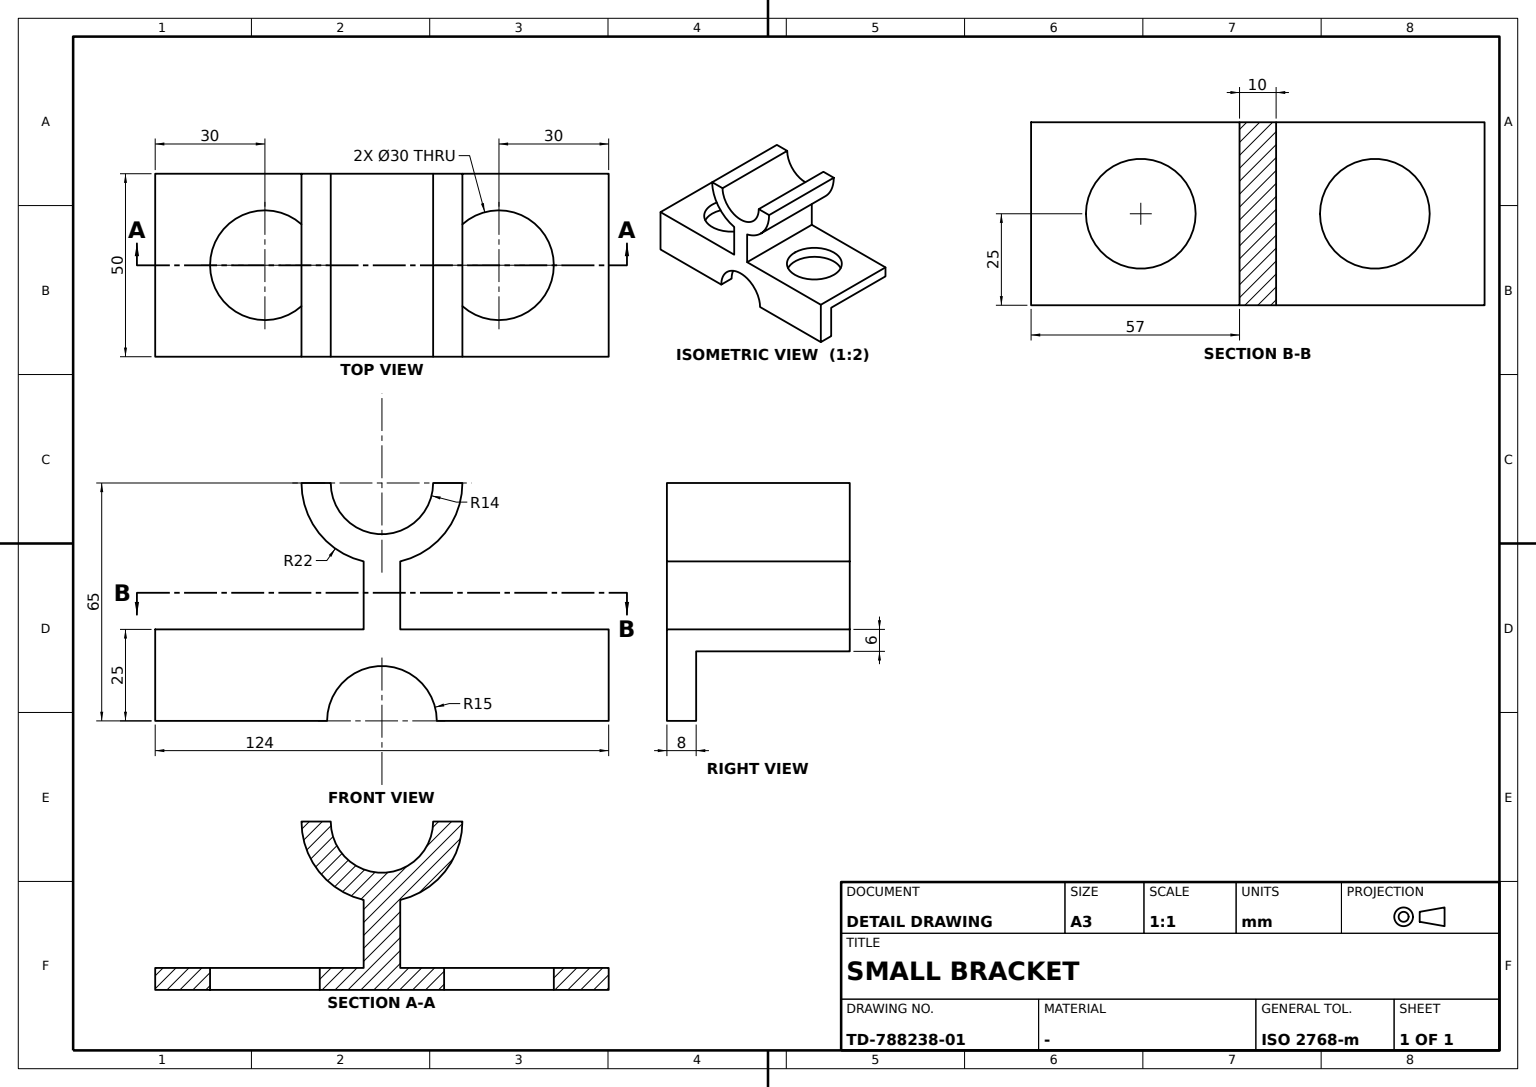
CATIA V5 part; units mm, degrees
sketch "Sketch1" plane through (0, 0, 0) normal (1, 0, 0) x (0, 1, 0)
  line L0 (0, 0) -> (0, 25)
  line L1 (0, 25) -> (50, 25)
  line L2 (50, 25) -> (50, 19)
  line L3 (50, 19) -> (8, 19)
  line L4 (8, 19) -> (8, 0)
  point P0 (8, 0)
  line L5 (8, 0) -> (0, 0)
  dimension "length L1" = 50
  dimension "length L2" = 6
  dimension "distance y axis L4" = 8
  dimension "distance L1 x axis" = 25
  constraint vertical L0 y-axis
  constraint vertical L2 y-axis
  constraint vertical L4 y-axis
  constraint horizontal L1 x-axis
  constraint horizontal L3 x-axis
  constraint horizontal L5 x-axis
  constraint coincidence P0 x-axis
extrude "Pad1" add sketch "Sketch1" along normal mid plane 124
sketch "Sketch2" plane through (0, 0, 0) normal (0, -1, 0) x (1, 0, 0)
  circle A0 centre (0, 0) radius 15
  dimension "radius A0" = 15
extrude "Pocket1" cut sketch "Sketch2" against normal up to next
sketch "Sketch3" plane through (0, 0, 0) normal (0, -1, 0) x (1, 0, 0)
  arc A0 (-14, 65) -> (14, 65) centre (0, 65) ccw
  point P0 (0, 65)
  arc A1 (-22, 65) -> (-5, 43.5757) centre (0, 65) ccw
  line L0 (-22, 65) -> (-14, 65)
  point P1 (14, 65)
  line L1 (14, 65) -> (22, 65)
  point P2 (-5, 25)
  line L2 (-5, 25) -> (-5, 43.5757)
  point P3 (-5, 43.5757)
  point P4 (5, 43.5757)
  point P5 (5, 25)
  line L3 (5, 25) -> (5, 43.5757)
  arc A2 (5, 43.5757) -> (22, 65) centre (0, 65) ccw
  line L4 (-5, 25) -> (5, 25)
  dimension "radius A0" = 14
  dimension "radius A1" = 22
  dimension "distance L3 L2" = 10
  constraint coincidence P0 y-axis
  constraint coincidence L0 P1
  constraint coincidence L0 P0
  constraint coincidence L0 L1
  constraint coincidence A1 A2
  constraint horizontal L0 x-axis
  constraint horizontal L1 x-axis
  constraint horizontal L4 x-axis
  constraint vertical L2 y-axis
extrude "Pad2" add sketch "Sketch3" against normal blind 50
sketch "Sketch4" plane through (38.5046, 10.6691, 25) normal (0, 0, 1) x (1, 0, 0)
  point P0 (-6.5046, 14.3309)
  line L0 (-100.5046, -10.6691) -> (23.4954, -10.6691) construction
  line L1 (23.4954, 39.3309) -> (23.4954, -10.6691) construction
  dimension "distance P0 L0" = 25
  dimension "distance P0 L1" = 30
hole "Hole1" at (32, 25, 25) direction (0, 0, -1) diameter 30 end up to next
mirror "Mirror1" about plane through (0, 0, 0) normal (1, 0, 0) of "Hole1"
properties part number "catia 17"
